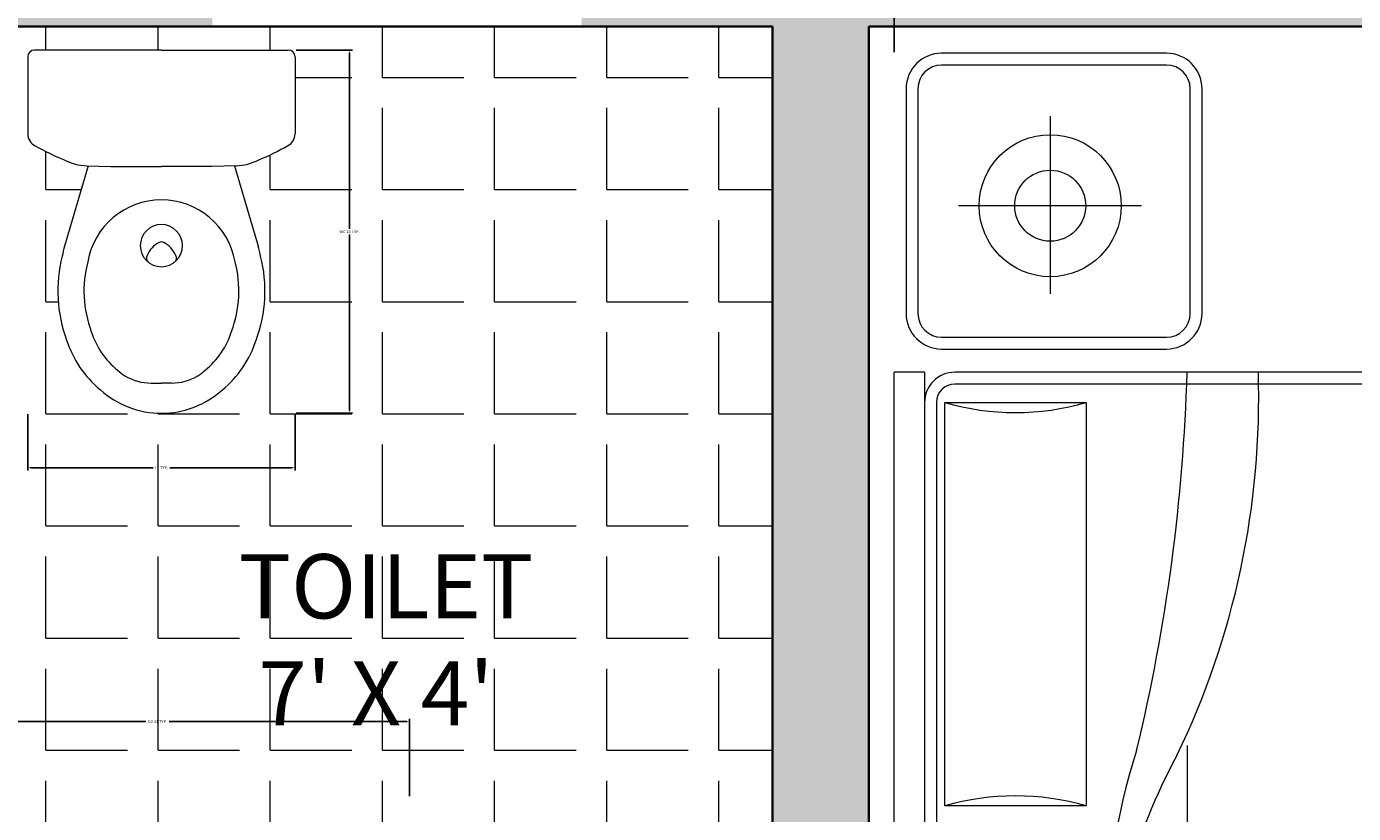
# Model space of a CAD drawing. Units: inches. Extents: x 2701 to 6846, y 811 to 2447.
# Tile 17 of 20: x 2926 to 3008, y 1407 to 1456. Entities that reach past the tile are written whole.
import ezdxf

# ---------------------------------------------------------------- set-up
doc = ezdxf.new("R2010")
doc.units = ezdxf.units.IN
for name, color, linetype, lineweight in [('A-ANNO-DIMS', 2, 'Continuous', 18), ('A-AREA-IDEN', 7, 'Continuous', 18), ('A-DOOR', 4, 'Continuous', 25), ('A-FLOR-FIXT', 7, 'Continuous', 18), ('A-FLOR-PATT', 252, 'Continuous', 13), ('A-FURN', 8, 'Continuous', 13), ('A-WALL', 7, 'Continuous', 35)]:
    doc.layers.add(name, color=color, linetype=linetype, lineweight=lineweight)
doc.layers.add('A-WALL-PATT', color=18, linetype='Continuous', lineweight=13, true_color=0x000000)
doc.styles.get("Standard").update_dxf_attribs({"font": 'arial.ttf'})
doc.dimstyles.get("Standard").update_dxf_attribs({"dimtxt": 0.18, "dimasz": 0.18, "dimexe": 0.18, "dimexo": 0.0625, "dimgap": 0.09, "dimtad": 0, "dimtih": 1, "dimtoh": 1, "dimdec": 4, "dimzin": 0, "dimdsep": 46, "dimtxsty": 'Standard', "dimcen": 0.09, "dimadec": 0, "dimazin": 0, "dimtfac": 1, "dimtdec": 4, "dimtofl": 0, "dimtmove": 0, "dimatfit": 3, "dimfxl": 1, "dimtolj": 1, "dimtzin": 0, "dimarcsym": 0})

# ---------------------------------------------------------------- blocks, each defined once
blk = doc.blocks.new('A$C356F0359')
for p, q in [((0.5488961549126543, 2.000037877005524), (2.049197857799299, 2.000037877005524)), ((2.049197857799299, 1.948857180890627), (2.049197857799299, 2.000037877005524)), ((2.528314948292972, 1.980067907948978), (2.148314948295592, 1.980067907948978)), ((2.528314948292972, 1.960067907952179), (2.148314948295592, 1.960067907952179)), ((2.049197857799299, 1.948857180890627), (0.5488961549126543, 1.948857180890627)), ((1.998017161684401, 1.928857180893828), (0.6000768510275521, 1.928857180893828)), ((2.088314948290644, 1.920067907951306), (2.088314948290644, 1.540067907953925)), ((2.108314948294719, 1.920067907951306), (2.108314948294719, 1.540067907953925)), ((2.568314948293846, 1.540067907953925), (2.568314948293846, 1.920067907951306)), ((2.588314948290644, 1.540067907953925), (2.588314948290644, 1.920067907951306)), ((2.029197857795224, 0.0512185731204227), (2.029197857795224, 1.897676484783005)), ((2.049197857799299, 0.0512185731204227), (2.049197857799299, 1.897676484783005)), ((2.330566813980112, 1.582168466462462), (2.330566813980112, 1.891729327624489)), ((2.481886725909134, 1.736603940531495), (2.181769094844639, 1.736603940531495)), ((2.148314948295592, 1.500067907953052), (2.528314948292972, 1.500067907953052)), ((2.148314948295592, 1.480067907948978), (2.528314948292972, 1.480067907948978))]:
    blk.add_line(p, q)
at = {"linetype": 'ByBlock'}
for p, q in [((1.316107238395488, 1.914736716818879), (1.998017161684401, 1.914736716818879)), ((1.316107238395488, 1.675893468294816), (1.316107238395488, 1.914736716818879)), ((1.998017161684401, 1.914736716818879), (1.998017161684401, 1.675893468294816)), ((1.998017161684401, 1.675893468294816), (1.316107238395488, 1.675893468294816)), ((1.418468630618008, 1.505291147914249), (0.5488961549126543, 1.505291147914249))]:
    blk.add_line(p, q, dxfattribs=at)
blk.add_circle((2.330566813980112, 1.736603940531495), 0.12, dxfattribs=at)
blk.add_circle((2.330566813980112, 1.736603940531495), 0.06)
for centre, radius, start, end in [((2.148314948295592, 1.920067907951306), 0.06, 90, 180), ((2.528314948292972, 1.920067907951306), 0.06, 0, 90), ((2.148314948295592, 1.920067907951306), 0.04, 90, 180), ((2.528314948292972, 1.920067907951306), 0.0399999999999709, 0, 90), ((1.998017161684401, 1.897676484783005), 0.0511806961126753, 0, 90), ((1.998017161684401, 1.897676484783005), 0.0311806961126753, 0, 90), ((2.148314948295592, 1.540067907953925), 0.06, 180, 270), ((2.148314948295592, 1.540067907953925), 0.04, 180, 270), ((2.528314948292972, 1.540067907953925), 0.06, 270, 0), ((2.528314948292972, 1.540067907953925), 0.04, 270, 0)]:
    blk.add_arc(centre, radius, start, end)
for centre, radius, start, end in [((0.9066616694908589, 1.795315092553209), 0.4265058009389605, 343.7397948414725, 16.26020515852748), ((2.407462730581755, 1.795315092553209), 0.4265058009389605, 163.7397948414725, 196.2602051585274), ((0.9302674239734187, 0.6570376961535658), 0.9852622038361044, 61.43284801268289, 88.12613015168571), ((1.082595312378543, 0.5712434438610217), 1.070619297177308, 72.19663287785316, 90.74183579771547), ((2.136771109289838, 4.599579859954246), 3.095527693941272, 256.4201152723854, 268.378871934336), ((2.005566012892813, 2.77448985040246), 1.390272332979946, 244.2426611098881, 271.7984468221989)]:
    blk.add_arc(centre, radius, start, end, dxfattribs=at)
blk = doc.blocks.new('A$C150B42AD')
at = {"ltscale": 20}
for p, q in [((0.2429999219411911, 0.6605010896237218), (0.0124999219360689, 0.6605010896237218)), ((0.2429999219411911, 0.6605010896237218), (0.4734999219390375, 0.6605010896237218)), ((-7.80610208e-08, 0.6480010896266322), (-7.80610208e-08, 0.5079979540751083)), ((0.4859999219361271, 0.6480010896266322), (0.4859999219361271, 0.5079979540751083)), ((0.1099663932354815, 0.4499086118448759), (0.0669662435202554, 0.3038111749119707)), ((0.1071200985052201, 0.4500080066427472), (0.1510932948976915, 0.4484724287904101)), ((0.1510932948976915, 0.4484724287904101), (0.2429999219411911, 0.4484724287904101)), ((0.3349065489774148, 0.4484724287904101), (0.2429999219411911, 0.4484724287904101)), ((0.3788797453698862, 0.4500080066427472), (0.3349065489774148, 0.4484724287904101)), ((0.3760334506469007, 0.4499086118448759), (0.419033600354851, 0.3038111749119707)), ((0.2244999219356032, 0.0549026304142899), (0.2429999219411911, 0.0549026304142899)), ((0.2614999219395031, 0.0549026304142899), (0.2429999219411911, 0.0549026304142899))]:
    blk.add_line(p, q, dxfattribs=at)
for centre, radius, start, end in [((0.0124999219360689, 0.6480010896266322), 0.0125, 90, 180), ((0.4734999219390375, 0.6480010896266322), 0.0125, 0, 90), ((0.0239999219365927, 0.5079979540751083), 0.024, 180, 243.9999999999169), ((0.4619999219385136, 0.5079979540751083), 0.024, 296.0000000000832, 0), ((0.2288323805723849, 0.861211124320107), 0.4322502624564528, 240.1180548737387, 247.8819451258213), ((0.2571674633099974, 0.861211124320107), 0.4322502624564528, 292.1180548741787, 299.8819451262613), ((0.1119175659141547, 0.5519209073245293), 0.1020257566424159, 243.3048371366711, 267.3048371363805), ((0.3740822779682276, 0.5519209073245293), 0.1020257566424159, 272.6951628636196, 296.6951628633288), ((0.2429999219411911, 0.2520000365038868), 0.1359999999999445, 90, 170.1093554438925), ((0.2429999219411911, 0.2520000365038868), 0.1359999999999054, 9.890644556107487, 90), ((0.2429999219411911, 0.3047433868632652), 0.0383668793900662, 90, 270), ((0.2429999219411911, 0.3047433868632652), 0.0383668793900662, 270, 90), ((0.2429999219411911, 0.2520000365038868), 0.1834999999995578, 163.5995179369745, 169.4685073238174), ((0.2644505607122483, 0.2649244167114375), 0.0524797911919514, 119.1738126186074, 155.015614861567), ((0.2438841986540865, 0.2978098350213258), 0.0138752344263254, 93.65396949145695, 111.1904535314196), ((0.2421156452282958, 0.2978098350213258), 0.0138752344263254, 68.80954646858042, 86.34603050854304), ((0.221549283162858, 0.2649244167114375), 0.0524797911919514, 24.98438513843297, 60.82618738139257), ((0.2429999219411911, 0.2520000365038868), 0.1834999999998773, 10.53149267661153, 16.40048206346955), ((0.3111168528876078, 0.2222454825459863), 0.2564589547706602, 165.7117968948095, 200.3376824053133), ((0.3111168528876078, 0.2222454825459863), 0.2089589547707847, 165.2744742501726, 200.6077610261089), ((0.2251027765405524, 0.2821865844234708), 0.0095725464836317, 149.1844377639907, 231.8077122469979), ((0.2608970673345539, 0.2821865844234708), 0.0095725464836317, 308.1922877530021, 30.81556223600924), ((0.1748829909874985, 0.2222454825459863), 0.2089589547707847, 339.3922389738912, 14.72552574982734), ((0.1748829909874985, 0.2222454825459863), 0.2564589547707392, 339.6623175946867, 14.28820310476077), ((0.2579999219406091, 0.1940000364993466), 0.1494999999998057, 197.6390904734559, 230.6281882087223), ((0.2279999219417732, 0.1940000364993466), 0.1494999999996299, 309.3718117912777, 342.360909526544), ((0.2579999219406091, 0.1940000364993466), 0.1969999999999626, 198.0034048038204, 230.2740437647753), ((0.2279999219417732, 0.1940000364993466), 0.1969999999999626, 309.7259562352247, 341.9965951961797), ((0.2429999219411911, 0.1660000365009182), 0.1184999999993879, 227.6454679706322, 235.8467474759224), ((0.2429999219411911, 0.1660000365009182), 0.1185000000000767, 304.1532525240776, 312.3545320293678), ((0.2244999219356032, 0.149902630415454), 0.0949999999999961, 239.6323803004523, 270), ((0.2614999219395031, 0.149902630415454), 0.0949999999999961, 270, 300.3676196995477), ((0.2429999219411911, 0.1660000365009182), 0.1660000000001673, 228.0788004750028, 270), ((0.2429999219411911, 0.1660000365009182), 0.16599999999994, 270, 311.9211995251523)]:
    blk.add_arc(centre, radius, start, end, dxfattribs=at)
blk = doc.blocks.new('DOOR-D2-30IN-PANEL-FRAME')
blk.add_lwpolyline([(-4.547e-13, 30.00000000000046), (-4.547e-13, 28.52062868157645), (4.3614931230818, 28.52062868157645), (4.3614931230818, 30.00000000000046), (-4.547e-13, 30.00000000000046)], close=True)
for points in [[(3.925343810773938, 30.00000000000046), (0.4361493129576957, 30.00000000000046)], [(4.361493123406944, 0), (4.361493123406944, 3.223968567697738), (31.40275048651847, 3.22396856790101), (31.40275048651847, 1.479371318667745), (1.623448e-10, 1.479371318424), (1.623448e-10, 0)], [(1.623448e-10, 0), (4.361493123406944, 0)], [(3.925343810773938, 0), (0.4361493129576957, 0)]]:
    blk.add_lwpolyline(points)
blk = doc.blocks.new('*D29')
at = {"layer": 'A-ANNO-DIMS', "color": 0, "lineweight": -2, "transparency": 16777216}
for p, q in [((2917.971391037054, 1408.112544742079), (2917.971391037054, 1412.940457315058)), ((2949.374141523573, 1408.112544742079), (2949.374141523573, 1412.940457315058)), ((2918.151391037054, 1412.760457315058), (2932.953502978813, 1412.760457315058)), ((2949.194141523573, 1412.760457315058), (2934.392029581814, 1412.760457315058))]:
    blk.add_line(p, q, dxfattribs=at)
at = {"layer": 'A-ANNO-DIMS', "color": 0, "transparency": 16777216}
for points in [[(2918.151391037054, 1412.790457315058), (2918.151391037054, 1412.730457315058), (2917.971391037054, 1412.760457315058)], [(2949.194141523573, 1412.790457315058), (2949.194141523573, 1412.730457315058), (2949.374141523573, 1412.760457315058)]]:
    blk.add_solid(points, dxfattribs=at)
at = {"layer": 'Defpoints', "color": 0, "transparency": 16777216}
for p in [(2949.374141523573, 1412.760457315058), (2917.971391037054, 1408.050044742079), (2949.374141523573, 1408.050044742079)]:
    blk.add_point(p, dxfattribs=at)
at = {"layer": 'A-ANNO-DIMS', "color": 0, "transparency": 16777216, "insert": (2933.672766280313, 1412.760457315058), "char_height": 0.18, "attachment_point": 5}
blk.add_mtext('\\A1;D2 31 TYP.', dxfattribs=at)
blk = doc.blocks.new('*D41')
at = {"layer": 'A-ANNO-DIMS', "color": 0, "lineweight": -2, "transparency": 16777216}
for p, q in [((2942.299753494797, 1454.588602992596), (2945.810413892828, 1454.588602992596)), ((2945.630413892828, 1454.408602992596), (2945.630413892828, 1443.461199301116)), ((2945.630413892828, 1432.147533672391), (2945.630413892828, 1443.094937363871)), ((2942.299753494797, 1431.967533672391), (2945.810413892828, 1431.967533672391))]:
    blk.add_line(p, q, dxfattribs=at)
at = {"layer": 'A-ANNO-DIMS', "color": 0, "transparency": 16777216}
for points in [[(2945.600413892828, 1454.408602992596), (2945.660413892829, 1454.408602992596), (2945.630413892828, 1454.588602992596)], [(2945.600413892828, 1432.147533672391), (2945.660413892829, 1432.147533672391), (2945.630413892828, 1431.967533672391)]]:
    blk.add_solid(points, dxfattribs=at)
at = {"layer": 'Defpoints', "color": 0, "transparency": 16777216}
for p in [(2942.237253494797, 1454.588602992596), (2945.630413892828, 1454.588602992596), (2942.237253494797, 1431.967533672391)]:
    blk.add_point(p, dxfattribs=at)
at = {"layer": 'A-ANNO-DIMS', "color": 0, "transparency": 16777216, "insert": (2945.630413892828, 1443.278068332492), "char_height": 0.18, "attachment_point": 5}
blk.add_mtext('\\A1;WC 23 TYP.', dxfattribs=at)
blk = doc.blocks.new('*D42')
at = {"layer": 'A-ANNO-DIMS', "color": 0, "lineweight": -2, "transparency": 16777216}
for p, q in [((2925.592556809366, 1431.90503367239), (2925.592556809366, 1428.394373274359)), ((2942.237253494795, 1431.90503367239), (2942.237253494795, 1428.394373274359)), ((2925.772556809366, 1428.57437327436), (2933.395287143895, 1428.57437327436)), ((2942.057253494795, 1428.57437327436), (2934.434523160267, 1428.57437327436))]:
    blk.add_line(p, q, dxfattribs=at)
at = {"layer": 'A-ANNO-DIMS', "color": 0, "transparency": 16777216}
for points in [[(2925.772556809366, 1428.60437327436), (2925.772556809366, 1428.54437327436), (2925.592556809366, 1428.57437327436)], [(2942.057253494795, 1428.60437327436), (2942.057253494795, 1428.54437327436), (2942.237253494795, 1428.57437327436)]]:
    blk.add_solid(points, dxfattribs=at)
at = {"layer": 'Defpoints', "color": 0, "transparency": 16777216}
for p in [(2925.592556809366, 1431.96753367239), (2942.237253494795, 1431.96753367239), (2942.237253494795, 1428.57437327436)]:
    blk.add_point(p, dxfattribs=at)
at = {"layer": 'A-ANNO-DIMS', "color": 0, "transparency": 16777216, "insert": (2933.914905152081, 1428.57437327436), "char_height": 0.18, "attachment_point": 5}
blk.add_mtext('\\A1;17 TYP.', dxfattribs=at)
blk = doc.blocks.new('*D52')
at = {"layer": 'A-ANNO-DIMS', "color": 0, "lineweight": -2, "transparency": 16777216}
for p, q in [((2979.552585764007, 1454.45252296757), (2979.552585764007, 1468.878707774448)), ((2979.732585764007, 1468.698707774448), (3016.218993565915, 1468.698707774448)), ((3053.141035747087, 1468.698707774448), (3016.654627945178, 1468.698707774448)), ((3053.321035747087, 1454.45252296757), (3053.321035747087, 1468.878707774448))]:
    blk.add_line(p, q, dxfattribs=at)
at = {"layer": 'A-ANNO-DIMS', "color": 0, "transparency": 16777216}
for points in [[(2979.732585764007, 1468.728707774448), (2979.732585764007, 1468.668707774448), (2979.552585764007, 1468.698707774448)], [(3053.141035747087, 1468.728707774448), (3053.141035747087, 1468.668707774448), (3053.321035747087, 1468.698707774448)]]:
    blk.add_solid(points, dxfattribs=at)
at = {"layer": 'Defpoints', "color": 0, "transparency": 16777216}
for p in [(2979.552585764007, 1468.698707774448), (2979.552585764007, 1454.39002296757), (3053.321035747087, 1454.39002296757)]:
    blk.add_point(p, dxfattribs=at)
at = {"layer": 'A-ANNO-DIMS', "color": 0, "transparency": 16777216, "insert": (3016.436810755547, 1468.698707774448), "char_height": 0.18, "attachment_point": 5}
blk.add_mtext('\\A1;74', dxfattribs=at)

msp = doc.modelspace()

# ---------------------------------------------------------------- hatches: boundary and pattern name
at = {"layer": 'A-FLOR-PATT'}
h = msp.add_hatch(dxfattribs=at)
h.set_pattern_fill('ANGLE', color=256)
h.set_pattern_definition([(0, (0, 0), (0, 6.985), [5.08, -1.905]), (90, (0, 0), (-6.985, 4e-16), [5.08, -1.905])])
h.paths.add_polyline_path([(2841.812531618507, 1296.510714093028, -0.1094531397224823), (2842.614165366529, 1300.128842847245, -0.1023747835315324), (2844.977063233859, 1303.301704019213, -0.0937428406070795), (2848.425874088265, 1305.367635711971, -0.0624630522953803), (2851.366818664733, 1306.050044742079), (2785.971391037217, 1306.050044742079), (2785.971391037217, 1258.050044742079), (2827.971391037217, 1258.050044742079), (2827.971391037217, 1256.411537864998), (2829.450762355621, 1256.411537864998, -0.3948265708167148), (2854.747422469505, 1283.452795228435), (2856.49201971855, 1283.452795228435), (2856.49201971876, 1256.411537865324), (2857.971391037219, 1256.411537865324), (2857.971391037219, 1258.05004474208), (2863.971391037218, 1258.050044742079), (2863.971391037217, 1306.050044742079), (2853.867060923166, 1306.050044742079, -0.0624630504647152), (2856.808005416599, 1305.367635742541, -0.0937428427235612), (2860.256816355725, 1303.301704017657, -0.1023747714125829), (2862.619714024758, 1300.128843269809, -0.1094531521575188), (2863.421347969692, 1296.510714138194, -0.109453153989093), (2862.619714017641, 1292.892584946142, -0.1023747709767553), (2860.256816355757, 1289.719724213534, -0.093738257087872), (2856.808189965141, 1287.653860434733, -0.0884250558281599), (2852.616939784454, 1286.906795737127, -0.0884250554332989), (2848.425689622791, 1287.653860434813, -0.0937382570330623), (2844.977063234018, 1289.719724212192, -0.1023747824199799), (2842.614165384649, 1292.892585345091, -0.1094531396555831)])
h.paths.add_polyline_path([(2805.214857085719, 1273.877134568363, -0.141745245190178), (2808.318689175414, 1271.772621468736, -0.1849834247598648), (2809.773740825251, 1267.974277286972, -0.1849834247688995), (2808.318689175285, 1264.175933105053, -0.141745244968364), (2805.214857091107, 1262.071420007333, -0.1522440861962393), (2799.994488829542, 1261.79557176336, -0.0256138964539793), (2799.368711507224, 1261.94541476925), (2794.365115778627, 1263.418098821323), (2794.36467071784, 1263.405353947873, -0.1112416791490392), (2793.99312620013, 1261.915170284834, -0.0338893268367682), (2793.114424873909, 1260.113565580275, -0.286745385218), (2792.375651823606, 1259.651928944151), (2787.580775843661, 1259.651928944133, -0.4142135623681101), (2787.152671505053, 1260.080033282747), (2787.152671505153, 1267.974277286972), (2787.152671505053, 1275.868521290948, -0.4142135623730951), (2787.580775843668, 1276.296625629562), (2792.375651823623, 1276.296625629544, -0.2867453846084762), (2793.114424873105, 1275.834988995069, -0.0338893268640583), (2793.99312620013, 1274.033384289111, -0.1051042356073151), (2794.361711671137, 1272.627936636842), (2794.365115778619, 1272.530455752619), (2799.368711507498, 1274.003139804786, -0.0256138965941945), (2799.994488833287, 1274.152982811292, -0.1522440859162748)], flags=16)
h.paths.add_polyline_path([(2804.681063364808, 1272.339952816459, -0.1449445299175104), (2807.087654609562, 1270.708506585421, -0.0358001151589041), (2807.447023191777, 1270.252713401882, -0.1332846890906797), (2807.893417732773, 1268.607871708063), (2807.893417732813, 1267.974277286972), (2807.893417732773, 1267.340682865632, -0.1332846888970446), (2807.447023193029, 1265.695841173949, -0.0358001152638917), (2807.087654609923, 1265.240047988954, -0.1449445297267833), (2804.681063368992, 1263.608601758809, -0.1554037438169349), (2800.343099481134, 1263.385728797012, -0.3645106918446579), (2796.485382154562, 1267.974277286972, -0.3645106920174053), (2800.343099483932, 1272.562825777418, -0.1554037435534987)], flags=0)
h.paths.add_polyline_path([(2800.015880108981, 1268.901471623875, 0.1692977046764319), (2799.131174998024, 1268.11576383613, 0.0766670309700064), (2799.100009657075, 1267.974277286936, 0.0766670313951798), (2799.13117499834, 1267.832790736999, 0.1692977045836763), (2800.015880108981, 1267.04708294982, 0.3052192884941762), (2800.365297210358, 1267.156497374013, 0.1695347489604994), (2800.650786991011, 1267.974277286972, 0.1695347391656343), (2800.365297241503, 1268.792057160761, 0.3052193300480048)], flags=0)
h.paths.add_polyline_path([(2971.971391037218, 1456.050044742079), (2923.971391037218, 1456.050044742079), (2923.971391037218, 1408.050044742079), (2922.332884160136, 1408.050044742079), (2922.332884160136, 1406.570673423676, -0.394826570816717), (2949.374141523573, 1381.274013309792), (2949.374141523573, 1379.529416060747), (2922.332884160461, 1379.529416060537), (2922.332884160461, 1378.050044742079), (2923.971391037218, 1378.050044742079), (2923.971391037217, 1372.050044742079), (2971.971391037217, 1372.050044742079)])
h.paths.add_polyline_path([(2939.8177624336, 1436.526417411941, -0.1417452451905352), (2937.713249333971, 1433.422585322236, -0.1849834247599418), (2933.914905152205, 1431.967533672398, -0.1849834247691276), (2930.116560970283, 1433.422585322367, -0.1417452449676952), (2928.01204787257, 1436.526417406529, -0.1522440861964963), (2927.736199628592, 1441.746785668103, -0.0256138964540868), (2927.886042634483, 1442.372562990423), (2929.358726686557, 1447.376158719022), (2929.345981813088, 1447.376603779809, -0.1112416791473441), (2927.855798150072, 1447.748148297517, -0.0338893268369074), (2926.054193445506, 1448.626849623741, -0.2867453852169366), (2925.592556809384, 1449.365622674043), (2925.592556809366, 1454.160498653989, -0.4142135623681173), (2926.020661147981, 1454.588602992596), (2933.914905152205, 1454.588602992496), (2941.809149156182, 1454.588602992596, -0.4142072303161659), (2942.237253494696, 1454.160507909187), (2942.237253494777, 1449.365622674043, -0.2867453846243844), (2941.775616860276, 1448.626849624529, -0.0338893268635044), (2939.974012154347, 1447.74814829752, -0.1051042356087532), (2938.568564502058, 1447.379562826511), (2938.471083617852, 1447.37615871903), (2939.943767670019, 1442.372562990154, -0.0256138965942444), (2940.093610676525, 1441.746785664364, -0.152244085915992)], flags=16)
h.paths.add_polyline_path([(2938.280580681695, 1437.060211132847, -0.1449445299182329), (2936.649134450649, 1434.653619888082, -0.0358001151583613), (2936.193341267117, 1434.294251305872, -0.1332846890907526), (2934.548499573297, 1433.847856764876), (2933.914905152205, 1433.847856764836), (2933.281310730865, 1433.847856764876, -0.1332846888976268), (2931.636469039176, 1434.294251304624, -0.0358001152630847), (2931.180675854191, 1434.653619887722, -0.14494452972667), (2929.549229624045, 1437.06021112865, -0.1554037438170702), (2929.326356662246, 1441.398175016512, -0.3645106918448713), (2933.914905152205, 1445.255892343087, -0.3645106920173691), (2938.503453642651, 1441.398175013717, -0.1554037435532691)], flags=0)
h.paths.add_polyline_path([(2969.158462562638, 1392.044508285666, -0.0937428443921736), (2971.224394311477, 1388.595697278927, -0.0884209696484748), (2971.971391037217, 1384.404631716083, -0.0884209680179829), (2971.224394332037, 1380.213566228077, -0.0937428458331012), (2969.158462561081, 1376.764755163806, -0.1023747798731684), (2965.985601516888, 1374.401857356678, -0.1094531425013952), (2962.367472681615, 1373.600223549837, -0.1094531553411192), (2958.74934344807, 1374.401857521223, -0.102374769792102), (2955.576482756955, 1376.764755163771, -0.0937382570879047), (2953.510618978154, 1380.213381554388, -0.0884250558281564), (2952.763554280548, 1384.404631735075, -0.0884250554336261), (2953.510618978239, 1388.595881896752, -0.0937382570324601), (2955.576482755607, 1392.044508285504, -0.1023747638736991), (2958.749343238892, 1394.40740583216, -0.10945316082308), (2962.367472636449, 1395.209039901022, -0.1094531494878097), (2965.985601690358, 1394.407406013345, -0.102374774975509)], flags=0)
edge = h.paths.add_edge_path(flags=16)
edge.add_arc((2961.074722408913, 1384.858947505427), 10.19921062335061, 20.21320321302568, 41.63359467655653, ccw=False)
edge.add_spline(control_points=[(2970.645798607602, 1388.382922212802), (2970.45927694694, 1387.830081875375), (2970.004018351208, 1386.480719475378), (2971.435235818619, 1384.395639569603), (2969.86804662324, 1382.338798369057), (2970.408139739579, 1381.010733700175), (2970.645798607602, 1380.426341238356)], knot_values=[0, 0, 0, 0, 0.0411087303528805, 0.1003374234737184, 0.1559132068848227, 0.1995857666183122, 0.1995857666183122, 0.1995857666183122, 0.1995857666183122], degree=3, periodic=0)
edge.add_arc((2961.074722408954, 1383.950315945844), 10.19921062335061, 318.3664053106646, 339.7867967863075, ccw=False)
edge.add_arc((2961.862292702369, 1383.250252100635), 9.145476143303874, 294.98529005245234, 318.3664053112933, ccw=False)
edge.add_arc((2962.367474738348, 1382.166141072693), 7.949438681384353, 269.9999862429006, 294.9853451035073, ccw=False)
edge.add_arc((2962.367470579714, 1382.166141072693), 7.949438681384465, 245.0146528606722, 270.00001621636034, ccw=False)
edge.add_arc((2962.872652615592, 1383.250252100682), 9.145476143303885, 221.633594689284, 245.0147081786685, ccw=False)
edge.add_arc((2963.660222908995, 1383.950315945905), 10.19921062335051, 200.2129623510071, 221.6335946899624, ccw=False)
edge.add_arc((2964.894158186733, 1384.404632705954), 11.5141250647146, 180.0000045856949, 200.2129623497761, ccw=False)
edge.add_arc((2964.894158186734, 1384.404630744956), 11.51412506471477, 159.7870376490639, 179.999994827515, ccw=False)
edge.add_arc((2963.660222908922, 1384.858947504804), 10.19921062335051, 138.3664053200289, 159.7870376464858, ccw=False)
edge.add_arc((2962.872652615694, 1385.559011350224), 9.145476143303881, 114.9852895697228, 138.3664053235114, ccw=False)
edge.add_arc((2962.367470579715, 1386.643122378167), 7.949438681384341, 89.99998624290072, 114.9853445481478, ccw=False)
edge.add_arc((2962.367474738348, 1386.643122378167), 7.949438681384461, 65.01465414332972, 90.00001621635698, ccw=False)
edge.add_arc((2961.862292702924, 1385.559011349966), 9.145476143303876, 41.63359468007258, 65.01470929671348, ccw=False)
h.paths.add_polyline_path([(2963.809881193461, 1393.327235568244, -0.1264579126559968), (2966.613496696745, 1390.682864813822, -0.1416969839114421), (2967.169431848072, 1388.76054773013), (2967.169431848171, 1387.405856218539, -1), (2969.570411442753, 1387.40585621857, -0.4142135626407067), (2968.369921644365, 1386.205366421279), (2963.567962456663, 1385.004876624353, 0.146217798515541), (2963.311249278865, 1384.663463983469), (2968.97016654397, 1385.639690083447), (2968.97016654397, 1383.154510596366), (2963.317428127216, 1384.129674263443, 0.1403115373898127), (2963.56796245605, 1383.804386826958), (2968.369921645561, 1382.603897029581, -0.4142135623489124), (2969.570411442753, 1381.403407232289, -1), (2967.169431848171, 1381.403407232289), (2967.169431848072, 1380.040463554169, -0.1490250791000606), (2966.557068512987, 1378.031526062613, -0.0127594246128423), (2966.264512020975, 1377.619349736432, -0.1063032105074506), (2963.809880694587, 1375.482028786924, -0.1268223860120219), (2961.166982861567, 1374.800713347196, -0.12682239841106), (2958.52408452876, 1375.482027883284, -0.1063031789236789), (2956.069454414507, 1377.619348785205, -0.0857220920089208), (2954.537253221299, 1380.622635309784, -0.0753510219692474), (2953.964044077883, 1384.404631725429, -0.0753510220208753), (2954.537253222076, 1388.186628143578, -0.0857220919249397), (2956.069454414099, 1391.189914665108, -0.1063031717113424), (2958.5240850283, 1393.327234664099, -0.1268223860250843), (2961.166982861567, 1394.008550103962, -0.1268223983642548)], flags=0)
h.paths.add_polyline_path([(2934.842099489099, 1441.725394388693, 0.1692977046741335), (2934.056391701355, 1442.610099499628, 0.0766670309649834), (2933.91490515217, 1442.641264840574, 0.0766670314095982), (2933.773418602207, 1442.610099499295, 0.1692977045780331), (2932.987710815057, 1441.72539438868, 0.305219290057435), (2933.097125240708, 1441.375977286128, 0.169534748594888), (2933.914905152205, 1441.090487506638, 0.1695347390414705), (2934.732685025499, 1441.375977255749, 0.3052193305973386)], flags=0)
h.paths.add_polyline_path([(2969.323819906164, 1387.40585621857, -1), (2967.416023384759, 1387.40585621857, -1)], flags=0)
h.paths.add_polyline_path([(2968.830636832988, 1387.40585621857, -1), (2967.909206457936, 1387.40585621857, -1)], flags=0)
h.paths.add_polyline_path([(2962.129657139981, 1384.357435236314, -1), (2960.208873464314, 1384.357435236314, -1)], flags=0)
h.paths.add_polyline_path([(2961.800868424529, 1384.357435236314, -1), (2960.537662179766, 1384.357435236314, -1)], flags=0)
h.paths.add_polyline_path([(2969.323819906164, 1381.403407232289, -1), (2967.416023384759, 1381.403407232289, -1)], flags=0)
h.paths.add_polyline_path([(2968.830636832988, 1381.403407232289, -1), (2967.909206457936, 1381.403407232289, -1)], flags=0)
h.paths.add_polyline_path([(3085.971391037217, 1306.050044742079), (3001.971391037217, 1306.050044742079), (3001.971391037217, 1300.050044742079), (3000.332884160462, 1300.050044742079), (3000.332884160462, 1298.570673423621), (3027.374141523574, 1298.570673423411), (3027.374141523574, 1296.826076174374, -0.3948265708167921), (3000.332884160137, 1271.529416060482), (3000.332884160137, 1270.050044742079), (3001.971391037216, 1270.050044742079), (3001.971391037217, 1258.050044742079), (3085.971391037217, 1258.050044742079)])
h.paths.add_polyline_path([(3033.332715044416, 1274.444953022308, -0.1023747723857111), (3035.695612729331, 1271.272092240373, -0.1094531510467398), (3036.49724665838, 1267.653963142847, -0.109453129065687), (3035.695613062762, 1264.035834715682, -0.102374792813879), (3033.332715044451, 1260.862973218194, -0.0937428491083937), (3029.883903848349, 1258.797041398739, -0.0884209654955001), (3025.692838473141, 1258.05004474208, -0.0884209669723455), (3021.501773032378, 1258.797041429867, -0.093742846952782), (3018.052961922706, 1260.862973216846, -0.1023747779170817), (3015.690064146835, 1264.035834192024, -0.1094531447948728), (3014.888430307195, 1267.653963097683, -0.1094531229044609), (3015.690063814699, 1271.272091335764, -0.1023747982671114), (3018.052961922546, 1274.444953023867, -0.0937382570344717), (3021.501588311451, 1276.510816801145, -0.0884250558280669), (3025.692838492134, 1277.25788149875, -0.0884250554332868), (3029.884088653796, 1276.510816801064, -0.0937382570874262)], flags=0)
edge = h.paths.add_edge_path(flags=16)
edge.add_arc((3026.847218107582, 1267.148783163603), 9.145476143303444, 24.985288685417686, 48.36640531129461, ccw=False)
edge.add_arc((3027.931329135525, 1267.653965199581), 7.949438681383711, -1.3757099395661498e-05, 24.98534353079839, ccw=False)
edge.add_arc((3027.931329135525, 1267.653961040948), 7.949438681383458, -24.98534255728248, 1.6216352207720774e-05, ccw=False)
edge.add_arc((3026.847218107536, 1268.159143076827), 9.145476143303622, 311.6335946892918, 335.0147121614734, ccw=False)
edge.add_arc((3026.147154262487, 1268.946713370386), 10.19921062335084, 290.21320321300624, 311.633594688656, ccw=False)
edge.add_spline(control_points=[(3029.671128969861, 1259.375637171695), (3029.086736508042, 1259.613296039718), (3027.758671839159, 1260.153389156057), (3025.701830638613, 1258.586199960678), (3023.616750732838, 1260.01741742809), (3022.267388332841, 1259.562158832357), (3021.714547995414, 1259.375637171695)], knot_values=[0, 0, 0, 0, 0.0436725597334895, 0.0992483431445938, 0.1584770362654316, 0.1995857666183122, 0.1995857666183122, 0.1995857666183122, 0.1995857666183122], degree=3, periodic=0)
edge.add_arc((3025.238522703413, 1268.946713370155), 10.19921062335076, 228.3664053199745, 249.78679678323948, ccw=False)
edge.add_arc((3024.538458857992, 1268.159143076927), 9.145476143303437, 204.9852869984493, 228.3664053234469, ccw=False)
edge.add_arc((3023.45434783005, 1267.65396104095), 7.949438681383719, 179.9999862429023, 204.9853415900221, ccw=False)
edge.add_arc((3023.454347830049, 1267.653965199583), 7.949438681383464, 155.0146544340279, 180.0000162163587, ccw=False)
edge.add_arc((3024.538458858251, 1267.148783164158), 9.14547614330361, 131.6335946800857, 155.0147095493943, ccw=False)
edge.add_arc((3025.238522702964, 1266.361212870303), 10.19921062335009, 110.2129623509966, 131.6335946778856, ccw=False)
edge.add_arc((3025.692839463013, 1265.127277592565), 11.51412506471423, 90.00000458569599, 110.2129623497689, ccw=False)
edge.add_arc((3025.692837502014, 1265.127277592564), 11.51412506471427, 69.78703764905441, 89.99999482750928, ccw=False)
edge.add_arc((3026.147154262372, 1266.361212870188), 10.19921062335108, 48.3664053106545, 69.78703764952758, ccw=False)
h.paths.add_polyline_path([(3032.478121424384, 1273.951981363762, -0.1063031716151077), (3034.615441420988, 1271.497350751304, -0.1268223860413822), (3035.296756861021, 1268.85445291773, -0.1268223983836015), (3034.615442325363, 1266.211554585404, -0.1063032176830601), (3032.478120473694, 1263.756923759752, -0.012759424397259), (3032.06594390682, 1263.464367621596, -0.1490250698458729), (3030.057006653981, 1262.852003931225), (3028.694062975896, 1262.852003931126, -0.4142135623806731), (3029.894552773218, 1261.651514133835, -1), (3027.493573178635, 1261.651514133737), (3026.293083381258, 1266.453473323247, 0.1403115373895235), (3025.967795944775, 1266.704007652081), (3026.94295961185, 1261.051269235327), (3024.457780124769, 1261.051269235327), (3025.434006224748, 1266.710186500432, 0.1462177985154153), (3025.092593583864, 1266.453473322634), (3023.892103786938, 1261.651514134932, -1.000000100073327), (3021.491124192355, 1261.651514133836, -0.4142135623731147), (3022.691613989647, 1262.852003931127), (3021.336922478021, 1262.852003931226, -0.1416970043012063), (3019.41460486282, 1263.407938240376, -0.1264579123471447), (3016.770235543815, 1266.211555085013, -0.1268223859959933), (3016.088920104255, 1268.854452917731, -0.1268223983918172), (3016.770234640404, 1271.497351250108, -0.1063031789240722), (3018.907555542179, 1273.951981364503, -0.0857220919129331), (3021.910842063079, 1275.484182556737, -0.0753510220530541), (3025.692838482788, 1276.057391701414, -0.075351022008823), (3029.474834900351, 1275.484182557402, -0.0857220920013936)], flags=0)
h.paths.add_polyline_path([(3072.364663406136, 1280.00178826655, -0.1849834247682267), (3076.163007588042, 1281.456839916512, -0.1849834247587431), (3079.961351769785, 1280.001788266685, -0.1417452451922909), (3082.065864869442, 1276.897956176945, -0.1522440859149591), (3082.341713112365, 1271.677587924556, -0.0256138965949624), (3082.191870105855, 1271.051810598748), (3080.719186053688, 1266.048214869872), (3080.816666937894, 1266.04481076239, -0.1051042356089094), (3082.222114590184, 1265.676225291381, -0.0338893268638024), (3084.023719296129, 1264.797523964363, -0.2867453846178035), (3084.485355930614, 1264.058750914859), (3084.485355930532, 1259.26388419012, -0.4142198944533688), (3084.057251592018, 1258.835770596306), (3076.163007588042, 1258.835770596406), (3068.268763583817, 1258.835770596306, -0.4142135623730951), (3067.840659245203, 1259.26387493492), (3067.84065924522, 1264.058750914876, -0.2867453852273427), (3068.302295881383, 1264.797523965184, -0.0338893268359893), (3070.103900585901, 1265.676225291382, -0.1051042356607345), (3071.509348238908, 1266.044810762424), (3071.606829122393, 1266.04821486988), (3070.134145070319, 1271.051810598479, -0.0256138964541135), (3069.984302064428, 1271.6775879208, -0.1522440861962023), (3070.260150308403, 1276.897956182364, -0.1417452449689107)], flags=16)
h.paths.add_polyline_path([(3073.428778290028, 1278.770753701179, -0.0358001152649927), (3073.884571475038, 1279.130122284293, -0.1332846888953009), (3075.529413166701, 1279.576516824026), (3076.163007588042, 1279.576516824066), (3076.796602009133, 1279.576516824026, -0.1332846890885353), (3078.441443702929, 1279.130122283046, -0.0358001151610664), (3078.897236886497, 1278.77075370081, -0.1449445299169966), (3080.528683117528, 1276.364162456064, -0.1554037435538929), (3080.751556078487, 1272.026198575177, -0.3645106920168784), (3076.163007588042, 1268.168481245816, -0.3645106918444272), (3071.574459098083, 1272.026198572385, -0.1554037438173037), (3071.797332059881, 1276.364162460253, -0.1449445297265802)], flags=0)
h.paths.add_polyline_path([(3026.700426809735, 1268.85217047715, -1), (3024.77964313407, 1268.85217047715, -1)], flags=0)
h.paths.add_polyline_path([(3026.371638094284, 1268.85217047715, -1), (3025.108431849521, 1268.85217047715, -1)], flags=0)
h.paths.add_polyline_path([(3075.268500788244, 1271.624470471877, 0.1576769337924287), (3076.021521038093, 1270.814274089584, 0.0766670314188588), (3076.163007588078, 1270.783108748328, 0.0766670308737057), (3076.3044941371, 1270.814274089222, 0.1576769338966524), (3077.057514387587, 1271.624470471873, 0.3746263233786361), (3076.980787467475, 1272.048396328269, 0.1695347405768383), (3076.163007588042, 1272.333886082264, 0.1695347491173554), (3075.345227674456, 1272.04839630111, 0.3746262855823952)], flags=0)
h.paths.add_polyline_path([(3029.64796123663, 1261.651514133835, -1), (3027.740164715224, 1261.651514133835, -1)], flags=0)
h.paths.add_polyline_path([(3029.154778163453, 1261.651514133835, -1), (3028.233347788401, 1261.651514133835, -1)], flags=0)
h.paths.add_polyline_path([(3023.645512250349, 1261.651514133836, -1), (3021.737715728944, 1261.651514133836, -1)], flags=0)
h.paths.add_polyline_path([(3023.152329177172, 1261.651514133836, -1), (3022.23089880212, 1261.651514133836, -1)], flags=0)
h.paths.add_polyline_path([(2810.572659831725, 1281.221625132062), (2833.310943898055, 1281.221625132062), (2833.310943898055, 1296.429027198873), (2810.572659831725, 1296.429027198873)], flags=24)
h.paths.add_polyline_path([(2937.545180300932, 1410.244315705433), (2960.208482391776, 1410.244315705433), (2960.208482391776, 1425.451717772244), (2937.545180300932, 1425.451717772244)], flags=24)
h.paths.add_polyline_path([(3043.227580059905, 1273.098575462184), (3065.890882150748, 1273.098575462184), (3065.890882150748, 1288.305977528995), (3043.227580059905, 1288.305977528995)], flags=24)
at = {"layer": 'A-WALL-PATT'}
h = msp.add_hatch(color=256, dxfattribs=at)
h.dxf.hatch_style = 1
h.paths.add_polyline_path([(3085.971391037218, 1456.050044742079), (3085.971391037217, 1348.050044742079), (3091.971391037218, 1348.050044742079), (3091.971391037218, 1360.050044742079), (3091.971391037218, 1462.050044742079), (2960.086244240269, 1462.050044742079), (2960.086244240269, 1456.050044742079), (2971.971391037218, 1456.050044742079), (2971.971391037217, 1372.050044742079), (2923.971391037217, 1372.050044742079), (2923.971391037218, 1378.050044742079), (2917.971391037217, 1378.050044742079), (2917.971391037217, 1351.050044742079), (2923.971391037218, 1351.050044742079), (2923.971391037217, 1366.050044742079), (2971.971391037218, 1366.050044742079), (2971.971391037218, 1351.05004474208), (2976.76903347243, 1351.05004474208), (2977.971391037218, 1351.050044742079), (2977.971391037218, 1456.050044742079)])
h.paths.add_polyline_path([(2779.971391037218, 1462.050044742079), (2779.971391037218, 1342.05004474208), (2785.971391037217, 1342.05004474208), (2785.971391037218, 1456.050044742079), (2917.971391037218, 1456.050044742079), (2917.971391037217, 1408.050044742079), (2922.332884160136, 1408.050044742079), (2923.971391037218, 1408.050044742079), (2923.971391037218, 1456.050044742079), (2937.086244240269, 1456.050044742079), (2937.086244240269, 1462.050044742079)])
h.paths.add_polyline_path([(2779.971391037217, 1306.050044742079), (2779.971391037217, 1294.241199564278), (2785.971391037217, 1294.241199564278), (2785.971391037217, 1306.050044742079), (2851.366818664733, 1306.050044742079, -0.0258153414615714), (2852.616939803445, 1306.114632493797, -0.0258153410699148), (2853.867060923166, 1306.050044742079), (2863.971391037217, 1306.050044742079), (2863.971391037218, 1258.050044742079), (2857.971391037219, 1258.05004474208), (2857.971391037218, 1252.050044742079), (2878.971391037217, 1252.050044742079), (2878.971391037217, 1258.050044742079), (2869.971391037218, 1258.050044742079), (2869.971391037217, 1306.050044742079), (2923.971391037217, 1306.050044742079), (2923.971391037218, 1318.050044742079), (2919.173748601648, 1318.050044742079), (2917.971391037216, 1318.050044742079), (2917.971391037216, 1312.050044742079), (2785.971391037217, 1312.050044742079), (2785.971391037217, 1318.050044742079), (2779.971391037217, 1318.050044742079)])
h.paths.add_polyline_path([(2785.971391037218, 1252.050044742079), (2827.971391037217, 1252.050044742079), (2827.971391037217, 1256.411537864998), (2827.971391037217, 1258.050044742079), (2785.971391037217, 1258.050044742079), (2785.971391037217, 1271.241199564278), (2779.971391037218, 1271.241199564278), (2779.971391037218, 1174.050044742079), (2785.971391037217, 1174.050044742079)])
h.paths.add_polyline_path([(2779.971391037218, 1030.050044742079), (2869.971391037218, 1030.050044742079), (2869.971391037218, 1036.050044742079), (2785.971391037218, 1036.050044742079), (2785.971391037217, 1126.050044742079), (2917.971391037217, 1126.050044742079), (2917.971391037216, 1120.050044742079), (2923.971391037218, 1120.050044742078), (2923.971391037218, 1258.050044742079), (2911.971391037217, 1258.050044742079), (2911.971391037217, 1253.252402306509), (2911.971391037218, 1252.050044742079), (2917.971391037218, 1252.050044742079), (2917.971391037217, 1132.050044742078), (2785.971391037217, 1132.050044742079), (2785.971391037217, 1144.050044742079), (2779.971391037218, 1144.050044742079)])
h.paths.add_polyline_path([(2935.971391037218, 1030.050044742079), (2935.971391037218, 1033.050044742079), (2935.971391037217, 1036.050044742079), (2923.971391037218, 1036.050044742079), (2923.971391037218, 1087.050044742077), (2919.173748602005, 1087.050044742077), (2917.971391037216, 1087.050044742079), (2917.971391037218, 1036.050044742079), (2893.971391037218, 1036.050044742079), (2893.971391037218, 1030.050044742079)])
h.paths.add_polyline_path([(2971.971391037218, 1036.050044742079), (2971.971391037218, 1030.050044742079), (3091.971391037218, 1030.050044742079), (3091.971391037218, 1060.050044742079), (3085.971391037217, 1060.050044742079), (3085.971391037217, 1036.050044742079)])
h.paths.add_polyline_path([(3085.971391037217, 1084.050044742079), (3091.971391037217, 1084.050044742079), (3091.971391037217, 1096.050044742079), (3091.971391037217, 1268.891476913671), (3085.971391037217, 1268.891476913671), (3085.971391037217, 1258.050044742079), (3001.971391037217, 1258.050044742079), (3001.971391037216, 1270.050044742079), (2995.971391037217, 1270.050044742079), (2995.971391037217, 1252.050044742079), (3085.971391037217, 1252.050044742079)])
h.paths.add_polyline_path([(3085.971391037217, 1306.050044742078), (3085.971391037217, 1291.891476913671), (3091.971391037218, 1291.891476913671), (3091.971391037218, 1318.050044742079), (3085.971391037217, 1318.050044742079), (3085.971391037217, 1312.050044742079), (2977.971391037218, 1312.050044742079), (2977.971391037217, 1318.050044742079), (2971.971391037218, 1318.050044742079), (2971.971391037218, 1306.050044742079), (2995.971391037217, 1306.050044742079), (2995.971391037217, 1300.050044742079), (3000.332884160462, 1300.050044742079), (3001.971391037217, 1300.050044742079), (3001.971391037217, 1306.050044742079)])

# ---------------------------------------------------------------- linework, layer by layer
at = {"layer": 'A-WALL'}
for p, q in [((2971.971391037217, 1456.050044742079), (2923.971391037218, 1456.050044742079)), ((2971.971391037217, 1372.050044742079), (2971.971391037218, 1456.050044742079)), ((3085.971391037219, 1456.050044742079), (2977.971391037218, 1456.050044742079)), ((2977.971391037218, 1351.050044742079), (2977.971391037218, 1456.050044742079))]:
    msp.add_line(p, q, dxfattribs=at)

# ---------------------------------------------------------------- block references
at = {"layer": 'A-DOOR'}
msp.add_blockref('DOOR-D2-30IN-PANEL-FRAME', (2917.971391037054, 1378.050044742079), dxfattribs=at)
at = {"layer": 'A-FLOR-FIXT', "xscale": 34.24834708915159, "yscale": 34.24834708915159, "zscale": 34.24834708915159}
msp.add_blockref('A$C150B42AD', (2925.592559482927, 1431.9675324223), dxfattribs=at)
at = {"layer": 'A-FURN', "xscale": 36.85134703248138, "yscale": 36.85134703248138, "zscale": 36.85134703248138, "rotation": 90}
msp.add_blockref('A$C356F0359', (3053.256675647645, 1359.007130578667), dxfattribs=at)

# ---------------------------------------------------------------- texts
at = {"layer": 'A-AREA-IDEN', "insert": (2938.723983473247, 1423.188559877507), "char_height": 4, "attachment_point": 1}
msp.add_mtext_dynamic_manual_height_columns("{\\fTimes New Roman|b0|i0|c0|p18;TOILET\\P 7' X 4'}", width=32.13606039491242, gutter_width=12.5, heights=[0], dxfattribs=at)

# ---------------------------------------------------------------- dimensions: what is measured, and where the dimension line sits
at = {"layer": 'A-ANNO-DIMS'}
dim = msp.add_linear_dim(base=(2979.552585764007, 1468.698707774448), p1=(3053.321035747087, 1454.39002296757), p2=(2979.552585764007, 1454.39002296757), angle=180, dimstyle='Standard', override={"dimdec": 0, "dimlfac": 1, "dimrnd": 0, "dimzin": 0, "dimdsep": 46, "dimlunit": 2}, dxfattribs=at)
dim.commit()
dim.dimension.update_dxf_attribs({"geometry": '*D52', "text_midpoint": (3016.436810755547, 1468.698707774448)})
dim = msp.add_linear_dim(base=(2945.630413892828, 1454.588602992596), p1=(2942.237253494795, 1431.96753367239), p2=(2942.237253494795, 1454.588602992595), angle=90, text='WC <> TYP.', dimstyle='Standard', override={"dimdec": 0, "dimlfac": 1, "dimrnd": 0, "dimzin": 0, "dimdsep": 46, "dimlunit": 2}, dxfattribs=at)
dim.commit()
dim.dimension.update_dxf_attribs({"geometry": '*D41', "text_midpoint": (2945.630413892828, 1443.278068332492)})
for base, p1, p2, text, picture, middle in [((2942.237253494795, 1428.57437327436), (2925.592556809366, 1431.96753367239), (2942.237253494795, 1431.96753367239), '<> TYP.', '*D42', (2933.914905152081, 1428.57437327436)), ((2949.374141523573, 1412.760457315058), (2917.971391037054, 1408.050044742079), (2949.374141523573, 1408.050044742079), 'D2 <> TYP.', '*D29', (2933.672766280313, 1412.760457315058))]:
    dim = msp.add_linear_dim(base=base, p1=p1, p2=p2, text=text, dimstyle='Standard', override={"dimdec": 0, "dimlfac": 1, "dimrnd": 0, "dimzin": 0, "dimdsep": 46, "dimlunit": 2}, dxfattribs=at)
    dim.commit()
    dim.dimension.update_dxf_attribs({"geometry": picture, "text_midpoint": middle})

doc.saveas('drawing.dxf')
